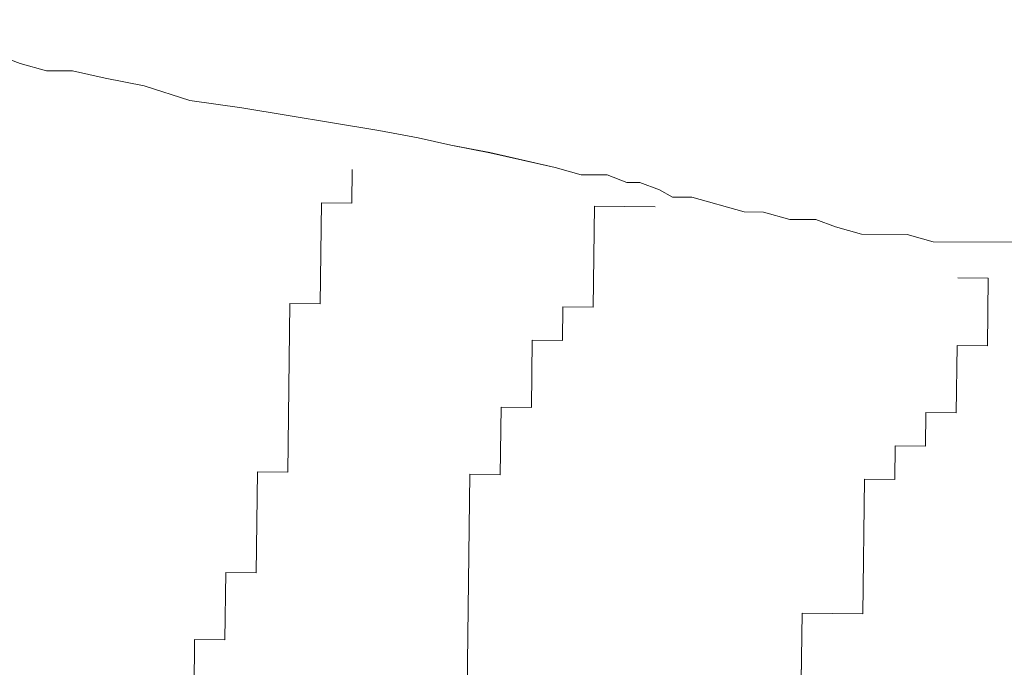
# Model space of a CAD drawing. Units: inches. Extents: x -466983 to 1020, y 324 to 318697.
# Tile 71 of 97: x 643.839 to 647.874, y 945.322 to 947.975. Entities that reach past the tile are written whole.
import ezdxf

# ---------------------------------------------------------------- set-up
doc = ezdxf.new("R2010")
doc.units = ezdxf.units.IN
doc.header["$MEASUREMENT"] = 0
doc.layers.add('A-FLOR-PATT', color=252, linetype='Continuous', lineweight=13)
doc.layers.add('A-FURN', color=8, linetype='Continuous', lineweight=18)

# ---------------------------------------------------------------- blocks, each defined once
blk = doc.blocks.new('L Shaped Sofa')
at = {"ltscale": 2}
for p, q in [((2415.2897, 737.5028), (2415.3174, 739.77)), ((2417.3467, 738.7374), (2417.3559, 739.4931)), ((2412.8069, 738.5409), (2412.813, 739.0447)), ((2417.1137, 738.2363), (2417.1198, 738.7401)), ((2417.1198, 738.7401), (2417.3467, 738.7374)), ((2412.3409, 737.5388), (2412.3532, 738.5464)), ((2412.3532, 738.5464), (2412.8069, 738.5409)), ((2416.8776, 737.4834), (2416.8868, 738.2391)), ((2416.8868, 738.2391), (2417.1137, 738.2363)), ((2412.111, 737.2896), (2412.114, 737.5416)), ((2412.114, 737.5416), (2412.3409, 737.5388)), ((2415.0568, 737.0017), (2415.0629, 737.5055)), ((2415.0629, 737.5055), (2415.2897, 737.5028)), ((2416.6354, 736.2266), (2416.6508, 737.4861)), ((2416.6508, 737.4861), (2416.8776, 737.4834)), ((2411.881, 737.0405), (2411.8841, 737.2924)), ((2411.8841, 737.2924), (2412.111, 737.2896)), ((2411.6481, 736.5394), (2411.6542, 737.0433)), ((2411.6542, 737.0433), (2411.881, 737.0405)), ((2414.8238, 736.5006), (2414.8299, 737.0045)), ((2414.8299, 737.0045), (2415.0568, 737.0017)), ((2411.4151, 736.0384), (2411.4212, 736.5422)), ((2411.4212, 736.5422), (2411.6481, 736.5394)), ((2414.5938, 736.2515), (2414.5969, 736.5034)), ((2414.5969, 736.5034), (2414.8238, 736.5006)), ((2414.3578, 735.4985), (2414.367, 736.2543)), ((2414.367, 736.2543), (2414.5938, 736.2515)), ((2416.3993, 735.4736), (2416.4085, 736.2293)), ((2416.4085, 736.2293), (2416.6354, 736.2266)), ((2411.6419, 736.0356), (2411.4151, 736.0384)), ((2410.4113, 735.7723), (2411.8264, 735.7657)), ((2411.8264, 735.7657), (2412.0212, 735.7106)), ((2412.0212, 735.7106), (2412.3628, 735.709)), ((2412.3628, 735.709), (2412.5576, 735.6538)), ((2412.5576, 735.6538), (2412.7037, 735.5989)), ((2412.7037, 735.5989), (2412.8989, 735.598)), ((2412.8989, 735.598), (2413.0937, 735.5429)), ((2413.0937, 735.5429), (2413.2401, 735.5422)), ((2413.2401, 735.5422), (2413.6298, 735.4319)), ((2413.9041, 735.5041), (2414.3578, 735.4985)), ((2416.1694, 735.2245), (2416.1725, 735.4764)), ((2416.1725, 735.4764), (2416.3993, 735.4736)), ((2413.6298, 735.4319), (2413.7762, 735.4312)), ((2413.7762, 735.4312), (2413.8734, 735.3766)), ((2413.8734, 735.3766), (2414.0195, 735.3217)), ((2414.0195, 735.3217), (2414.1171, 735.3212)), ((2414.1171, 735.3212), (2414.2631, 735.2663)), ((2414.2631, 735.2663), (2414.4583, 735.2654)), ((2414.4583, 735.2654), (2414.6532, 735.2103)), ((2414.6532, 735.2103), (2415.1404, 735.0995)), ((2415.1404, 735.0995), (2415.4329, 735.0439)), ((2415.4329, 735.0439), (2415.6765, 734.9886)), ((2415.6765, 734.9886), (2415.969, 734.933)), ((2415.969, 734.933), (2416.9927, 734.7655)), ((2416.9927, 734.7655), (2417.3827, 734.7095)), ((2417.3827, 734.7095), (2417.7236, 734.5994)), ((2417.7236, 734.5994), (2418.016, 734.5439)), ((2418.016, 734.5439), (2418.2597, 734.4885)), ((2418.2597, 734.4885), (2418.4549, 734.4876)), ((2418.4549, 734.4876), (2418.6497, 734.4324)), ((2418.6497, 734.4324), (2418.7958, 734.3775))]:
    blk.add_line(p, q, dxfattribs=at)

msp = doc.modelspace()

# ---------------------------------------------------------------- hatches: boundary and pattern name
at = {"layer": 'A-FLOR-PATT', "transparency": 33554572}
h = msp.add_hatch(dxfattribs=at)
h.set_pattern_fill('ANSI37', color=256, scale=30)
h.set_pattern_definition([(45, (-1212.4137, -290.035), (-2.6516504, 2.6516504), []), (135, (-1212.4137, -290.035), (-2.6516504, -2.6516504), [])])
h.paths.add_polyline_path([(901.8057, 1075.9377), (900.6144, 1075.9377), (900.6144, 1065.3856), (899.391, 1065.3856), (898.0911, 1065.3856), (892.8356, 1058.7098, -0.258377), (892.1875, 1058.3509), (879.9848, 1058.3509, -0.20177), (879.4382, 1058.5808), (874.0812, 1065.3856), (872.7813, 1065.3856), (871.5579, 1065.3856), (871.5579, 1075.9377), (813.8057, 1075.9377), (813.8057, 1044.7922), (832.3947, 1044.7922, -0.394795), (848.6602, 1028.5356), (848.6602, 1009.9377), (901.8057, 1009.9377), (901.8057, 1015.9377), (901.3057, 1015.9377), (871.3057, 1015.9377), (871.3057, 1017.2502), (871.3344, 1017.2502, -0.401453), (901.3057, 1045.9377), (901.8057, 1045.9377)])
edge = h.paths.add_edge_path(flags=16)
edge.add_line((847.7731, 1068.9486), (847.7731, 1073.7088))
edge.add_arc((849.2269, 1073.7088), 1.4538, 90, 180, ccw=False)
edge.add_line((849.2269, 1075.1627), (864.4921, 1075.1627))
edge.add_arc((864.4921, 1073.7088), 1.4538, 0, 90, ccw=False)
edge.add_line((865.9459, 1073.7088), (865.9459, 1069.0035))
edge.add_arc((832.6447, 1068.9761), 33.3012, -20.61234, 0.04725, ccw=False)
edge.add_ellipse((856.8595, 1058.48), major_axis=(0, 10.2131), ratio=0.6859192, start_angle=100.00884, end_angle=259.99116, ccw=False)
edge.add_arc((881.0742, 1068.9761), 33.3012, 180.04725, 200.61234, ccw=False)
h.paths.add_polyline_path([(853.1456, 1066.4815), (853.1456, 1066.4534), (853.1463, 1066.4534, 0.433107), (852.9166, 1066.6849), (852.9166, 1066.4534), (853.1456, 1066.4534), (853.1456, 1066.4815), (853.088, 1066.6122, 0.697939), (852.6995, 1066.4534), (852.7003, 1066.4534), (852.7003, 1066.4815), (852.9166, 1067.0012), (852.9166, 1066.6849, -0.396254)], flags=0)
h.paths.add_polyline_path([(861.0187, 1066.4815), (861.0187, 1066.4534), (861.0194, 1066.4534, 0.416404), (860.8024, 1066.6849), (860.8024, 1066.4534), (861.0187, 1066.4534), (861.0187, 1066.4815), (860.9672, 1066.6053, 0.713344), (860.5726, 1066.4534), (860.5734, 1066.4534), (860.5734, 1066.4815), (860.8024, 1067.0012), (860.8024, 1066.6849, -0.379973)], flags=0)
edge = h.paths.add_edge_path(flags=0)
edge.add_spline(control_points=[(861.1298, 1065.7855), (861.4661, 1065.2478), (861.6134, 1065.0161), (861.9833, 1064.3736), (862.1924, 1063.9443), (862.5614, 1063.0391), (862.7212, 1062.5633), (862.9865, 1061.5781), (863.092, 1061.0689), (863.2452, 1060.031), (863.293, 1059.5025), (863.3295, 1058.4409), (863.3181, 1057.9078), (863.2366, 1056.8518), (863.1664, 1056.3289), (862.9695, 1055.308), (862.8427, 1054.8099), (862.5365, 1053.8522), (862.3571, 1053.3927), (861.9514, 1052.5249), (861.7251, 1052.1166), (861.233, 1051.3622), (860.9672, 1051.0162), (860.4048, 1050.3949), (860.1082, 1050.1197), (859.4937, 1049.6461), (859.1758, 1049.4476), (858.5276, 1049.1299), (858.1973, 1049.0107), (857.5315, 1048.8518), (857.1959, 1048.8121), (856.5249, 1048.812), (856.1894, 1048.8515), (855.5236, 1049.0101), (855.1933, 1049.1291), (854.545, 1049.4465), (854.2271, 1049.6449), (853.6124, 1050.1183), (853.3158, 1050.3933), (852.7533, 1051.0143), (852.4874, 1051.3602), (851.9952, 1052.1144), (851.7688, 1052.5225), (851.3629, 1053.3902), (851.1834, 1053.8496), (850.877, 1054.8071), (850.7501, 1055.3051), (850.553, 1056.326), (850.4827, 1056.8488), (850.401, 1057.9048), (850.3895, 1058.4379), (850.4257, 1059.4995), (850.4734, 1060.0281), (850.6265, 1061.066), (850.7318, 1061.5753), (850.9969, 1062.5605), (851.1567, 1063.0365), (851.5254, 1063.9418), (851.7345, 1064.3712), (852.1056, 1065.0164), (852.2544, 1065.2503), (852.6082, 1065.7335)], knot_values=[3.915332, 3.915332, 3.915332, 3.915332, 4.013468, 4.013468, 4.175532, 4.175532, 4.337596, 4.337596, 4.49966, 4.49966, 4.661724, 4.661724, 4.823788, 4.823788, 4.985852, 4.985852, 5.147916, 5.147916, 5.30998, 5.30998, 5.472044, 5.472044, 5.634109, 5.634109, 5.796173, 5.796173, 5.958237, 5.958237, 6.120301, 6.120301, 6.282365, 6.282365, 6.444429, 6.444429, 6.606493, 6.606493, 6.768557, 6.768557, 6.930621, 6.930621, 7.092685, 7.092685, 7.254749, 7.254749, 7.416813, 7.416813, 7.578878, 7.578878, 7.740942, 7.740942, 7.903006, 7.903006, 8.06507, 8.06507, 8.227134, 8.227134, 8.389198, 8.389198, 8.551262, 8.551262, 8.65037, 8.65037, 8.65037, 8.65037], degree=3, periodic=0)
edge.add_line((852.6421, 1065.7855), (861.1298, 1065.7855))
edge = h.paths.add_edge_path(flags=0)
edge.add_ellipse((856.8496, 1057.7432), major_axis=(0, 7.7921), ratio=0.687861, start_angle=0, end_angle=360)
h.paths.add_polyline_path([(848.8634, 1069.3891), (848.8634, 1073.9605, -0.414214), (849.9538, 1075.0508), (863.7652, 1075.0508, -0.414214), (864.8555, 1073.9605), (864.8555, 1069.3891, -0.388936), (864.5237, 1069.027, -0.043561), (849.1953, 1069.027, -0.388936)], flags=0)
h.paths.add_polyline_path([(853.1006, 1068.1122, -1), (852.6775, 1068.1122, -1)], flags=0)
edge = h.paths.add_edge_path(flags=0)
edge.add_ellipse((856.8595, 1057.3378), major_axis=(0, 2.207), ratio=0.657164, start_angle=0, end_angle=360)
h.paths.add_polyline_path([(861.0415, 1068.1122, -1), (860.6184, 1068.1122, -1)], flags=0)
edge = h.paths.add_edge_path()
edge.add_line((573.9537, 1057.3412), (573.9537, 1075.9377))
edge.add_line((573.9537, 1075.9377), (558.7308, 1075.9377))
edge.add_line((558.7308, 1075.9377), (558.7308, 1065.3856))
edge.add_line((558.7308, 1065.3856), (557.5074, 1065.3856))
edge.add_line((557.5074, 1065.3856), (556.2075, 1065.3856))
edge.add_line((556.2075, 1065.3856), (550.952, 1058.7098))
edge.add_arc((550.3039, 1059.1155), 0.7646, 270, 327.9483, ccw=False)
edge.add_line((550.3039, 1058.3509), (538.1012, 1058.3509))
edge.add_arc((538.1012, 1059.1155), 0.7646, 224.3704, 270, ccw=False)
edge.add_line((537.5546, 1058.5808), (532.1976, 1065.3856))
edge.add_line((532.1976, 1065.3856), (530.8977, 1065.3856))
edge.add_line((530.8977, 1065.3856), (529.6743, 1065.3856))
edge.add_line((529.6743, 1065.3856), (529.6743, 1075.9377))
edge.add_line((529.6743, 1075.9377), (520.8057, 1075.9377))
edge.add_line((520.8057, 1075.9377), (520.8057, 1045.9377))
edge.add_line((520.8057, 1045.9377), (521.3057, 1045.9377))
edge.add_arc((521.3057, 1015.9377), 30, 2.50749, 90, ccw=False)
edge.add_line((551.277, 1017.2502), (551.3057, 1017.2502))
edge.add_line((551.3057, 1017.2502), (551.3057, 1015.9377))
edge.add_line((551.3057, 1015.9377), (520.8057, 1015.9377))
edge.add_line((520.8057, 1015.9377), (520.8057, 1009.9377))
edge.add_line((520.8057, 1009.9377), (559.1913, 1010.4022))
edge.add_arc((559.1913, 1011.856), 1.4538, 180, 270, ccw=False)
edge.add_line((557.7375, 1011.856), (557.7375, 1016.5613))
edge.add_arc((591.0386, 1016.5888), 33.3012, 159.38766, 180.04725, ccw=False)
edge.add_ellipse((566.8239, 1027.0848), major_axis=(0, 10.2131), ratio=0.6859192, start_angle=280.00884, end_angle=439.99116, ccw=False)
edge.add_arc((542.6091, 1016.5888), 33.3012, 0.04725, 20.61234, ccw=False)
edge.add_line((575.9103, 1016.6162), (575.9103, 1011.856))
edge.add_arc((574.4565, 1011.856), 1.4538, -90, 0, ccw=False)
edge.add_line((574.4565, 1010.4022), (608.8057, 1009.9377))
edge.add_line((608.8057, 1009.9377), (608.8057, 1041.0857))
edge.add_line((608.8057, 1041.0857), (590.2179, 1041.0857))
edge.add_arc((590.775, 1057.9074), 16.8309, 181.92775, 268.10321, ccw=False)
edge = h.paths.add_edge_path()
edge.add_ellipse((494.2443, 583.6204), major_axis=(0, 10.2131), ratio=0.6859192, start_angle=280.00884, end_angle=439.99116, ccw=False)
edge.add_arc((470.0296, 573.1243), 33.3012, 0.04725, 20.61234, ccw=False)
edge.add_line((503.3307, 573.1518), (503.3307, 568.3916))
edge.add_arc((501.8769, 568.3916), 1.4538, -90, 0, ccw=False)
edge.add_line((501.8769, 566.9377), (539.8057, 566.9377))
edge.add_line((539.8057, 566.9377), (539.8057, 572.9377))
edge.add_line((539.8057, 572.9377), (539.3057, 572.9377))
edge.add_line((539.3057, 572.9377), (509.3057, 572.9377))
edge.add_line((509.3057, 572.9377), (509.3057, 574.2502))
edge.add_line((509.3057, 574.2502), (509.3344, 574.2502))
edge.add_arc((539.3057, 572.9377), 30, 90, 177.49251, ccw=False)
edge.add_line((539.3057, 602.9377), (539.8057, 602.9377))
edge.add_line((539.8057, 602.9377), (539.8057, 626.9377))
edge.add_line((539.8057, 626.9377), (531.7718, 626.9377))
edge.add_line((531.7718, 626.9377), (531.7718, 616.3856))
edge.add_line((531.7718, 616.3856), (530.5484, 616.3856))
edge.add_line((530.5484, 616.3856), (529.2485, 616.3856))
edge.add_line((529.2485, 616.3856), (523.7105, 609.3509))
edge.add_line((523.7105, 609.3509), (510.7766, 609.3509))
edge.add_line((510.7766, 609.3509), (505.2386, 616.3856))
edge.add_line((505.2386, 616.3856), (503.9387, 616.3856))
edge.add_line((503.9387, 616.3856), (502.7153, 616.3856))
edge.add_line((502.7153, 616.3856), (502.7153, 626.9377))
edge.add_line((502.7153, 626.9377), (481.6983, 626.9377))
edge.add_line((481.6983, 626.9377), (481.6983, 610.995))
edge.add_arc((467.2703, 611.4728), 14.4359, 271.92775, 358.10321, ccw=False)
edge.add_line((467.7559, 597.0451), (451.8057, 597.0451))
edge.add_line((451.8057, 597.0451), (451.8057, 584.4035))
edge.add_line((451.8057, 584.4035), (451.8057, 566.9377))
edge.add_line((451.8057, 566.9377), (486.6117, 566.9377))
edge.add_arc((486.6117, 568.3916), 1.4538, 180, 270, ccw=False)
edge.add_line((485.1579, 568.3916), (485.1579, 573.0969))
edge.add_arc((518.4591, 573.1243), 33.3012, 159.38766, 180.04725, ccw=False)
h.paths.add_polyline_path([(836.2609, 1020.7328), (879.8898, 1020.7328), (879.8898, 1039.3902), (836.2609, 1039.3902)], flags=25)
h.paths.add_polyline_path([(549.9851, 1036.7492), (593.614, 1036.7492), (593.614, 1055.4065), (549.9851, 1055.4065)], flags=24)
h.paths.add_polyline_path([(475.123, 595.5959), (518.752, 595.5959), (518.752, 614.2532), (475.123, 614.2532)], flags=24)
h = msp.add_hatch(dxfattribs=at)
h.set_pattern_fill('ANSI37', color=256, scale=20)
h.set_pattern_definition([(45, (-1212.4137, -290.035), (-1.767767, 1.767767), []), (135, (-1212.4137, -290.035), (-1.767767, -1.767767), [])])
h.paths.add_polyline_path([(809.8057, 870.9377), (809.8057, 888.1519), (806.9985, 888.1519), (802.6624, 888.1519), (789.3832, 888.1519), (786.2846, 888.1519, -0.414214), (785.4991, 888.9374), (785.4991, 900.1959), (785.4991, 908.4696, -0.414214), (786.8082, 909.7787, -0.414214), (785.4991, 911.0878), (785.4991, 929.1015, -0.414214), (786.8082, 930.4106, -0.414214), (785.4991, 931.7197), (785.4991, 931.9039, -0.414214), (784.19, 930.5948), (766.7223, 930.5948, -0.412359), (765.4132, 931.8956, -0.413741), (764.1145, 930.5782), (744.5781, 930.422, -0.416556), (743.7864, 931.2075), (743.7864, 933.5153), (742.2154, 933.5153), (742.2154, 952.024, -0.001344), (743.7864, 952.1998), (743.7864, 953.9377), (678.5915, 953.9377), (678.5915, 951.1305), (678.5915, 946.7945), (678.5915, 933.5153), (678.5915, 930.4166, -0.414214), (677.806, 929.6312), (666.5475, 929.6312), (658.2738, 929.6312, -0.414214), (656.9647, 930.9403, -0.414214), (655.6556, 929.6312), (637.6419, 929.6312, -0.414214), (636.3328, 930.9403, -0.414214), (635.0237, 929.6312), (634.8395, 929.6312, -0.414214), (636.1486, 928.322), (636.1486, 910.8544, -0.412359), (634.8478, 909.5452, -0.413741), (636.1653, 908.2466), (636.3214, 888.7102, -0.416556), (635.5359, 887.9184), (633.2281, 887.9184), (633.2281, 886.3475), (614.7194, 886.3475, -0.001344), (614.5436, 887.9184), (612.8057, 887.9184), (612.8057, 834.9377), (612.8057, 752.9377), (612.8057, 748.9377), (612.8057, 697.9377), (654.8057, 697.9377), (654.8057, 701.9377), (715.8057, 701.9377), (715.8057, 737.4353), (774.2918, 737.4353), (774.2918, 795.9377), (809.8057, 795.9377)])
h.paths.add_polyline_path([(679.2761, 849.5757, 0.102523), (682.1475, 849.2608, -0.080461), (694.5428, 849.7725, -0.283899), (694.4822, 849.0082, 0.136605), (694.4068, 848.8103, -0.030441), (694.5428, 846.8929), (694.5428, 842.6198), (694.5428, 838.3466, -0.028219), (694.4246, 836.5684), (694.425, 836.5684, 0.196187), (694.4456, 836.2708, -0.302897), (694.5428, 835.467, -0.080461), (682.1475, 835.9787, 0.102523), (679.2761, 835.6638, -0.58611), (678.6457, 836.0169), (678.6457, 849.2227, -0.58611)], flags=16)
h.paths.add_polyline_path([(679.5173, 848.6515, 0.699597), (679.476, 848.6342, 1.20716), (679.1935, 848.7422, 0.010621)], flags=0)
h.paths.add_polyline_path([(679.4923, 836.5608, -0.013798), (679.9178, 836.6594, -0.071703), (682.8533, 837.1434, -0.165743), (682.1665, 839.1006), (682.1665, 842.6094), (682.1665, 846.0603, -0.240616), (683.4733, 848.6767, -0.068263), (693.9295, 849.0082), (693.7875, 848.7083), (693.7875, 849.0228, 0.067332), (683.4733, 848.6767, 0.240616), (682.1665, 846.0603), (682.1665, 842.6094), (682.1665, 839.1006, 0.23459), (683.461, 836.5513, 0.068093), (693.7875, 836.1955), (693.7875, 836.5104), (693.9296, 836.2102, -0.077215), (682.2421, 836.7815, 0.086627), (679.5283, 836.5701, -0.628402), (679.5029, 836.5735), (679.5029, 836.6071, 0.910458)], flags=0)
h.paths.add_polyline_path([(679.476, 848.6364), (679.2069, 848.647), (679.2069, 836.5718, 0.913566), (679.3645, 836.5861), (679.476, 836.5824)], flags=0)
h.paths.add_polyline_path([(679.2761, 829.8604, 0.102523), (682.1475, 829.5455, -0.080461), (694.5428, 830.0572, -0.283899), (694.4822, 829.2929, 0.136605), (694.4068, 829.095, -0.030441), (694.5428, 827.1776), (694.5428, 822.9045), (694.5428, 818.6314, -0.028219), (694.4246, 816.8531), (694.425, 816.8532, 0.196187), (694.4456, 816.5555, -0.302897), (694.5428, 815.7517, -0.080461), (682.1475, 816.2635, 0.102523), (679.2761, 815.9485, -0.58611), (678.6457, 816.3016), (678.6457, 829.5074, -0.58611)], flags=16)
h.paths.add_polyline_path([(679.5173, 828.9362, 0.699597), (679.476, 828.9189, 1.20716), (679.1935, 829.0269, 0.010621)], flags=0)
h.paths.add_polyline_path([(679.4923, 816.8456, -0.013798), (679.9178, 816.9441, -0.071703), (682.8533, 817.4281, -0.165743), (682.1665, 819.3853), (682.1665, 822.8941), (682.1665, 826.345, -0.240616), (683.4733, 828.9614, -0.068263), (693.9295, 829.2929), (693.7875, 828.9931), (693.7875, 829.3076, 0.067332), (683.4733, 828.9614, 0.240616), (682.1665, 826.345), (682.1665, 822.8941), (682.1665, 819.3853, 0.23459), (683.461, 816.836, 0.068093), (693.7875, 816.4802), (693.7875, 816.7952), (693.9296, 816.4949, -0.077215), (682.2421, 817.0662, 0.086627), (679.5283, 816.8549, -0.628402), (679.5029, 816.8582), (679.5029, 816.8918, 0.910458)], flags=0)
h.paths.add_polyline_path([(679.476, 828.9211), (679.2069, 828.9317), (679.2069, 816.8565, 0.913566), (679.3645, 816.8708), (679.476, 816.8671)], flags=0)
h.paths.add_polyline_path([(679.2761, 810.1451, 0.102523), (682.1475, 809.8302, -0.080461), (694.5428, 810.342, -0.3023), (694.4466, 809.5394, 0.10023), (694.4058, 809.3878, -0.03057), (694.5428, 807.4623), (694.5428, 803.1892), (694.5428, 798.9161, -0.03057), (694.4058, 796.9906, 0.10023), (694.4466, 796.839, -0.3023), (694.5428, 796.0365, -0.080461), (682.1475, 796.5482, 0.102523), (679.2761, 796.2333, -0.58611), (678.6457, 796.5863), (678.6457, 809.7921, -0.58611)], flags=16)
h.paths.add_polyline_path([(679.5173, 809.2417, 0.699597), (679.476, 809.2244, 1.20716), (679.1935, 809.3324, 0.010621)], flags=0)
h.paths.add_polyline_path([(679.4923, 797.151, -0.013798), (679.9178, 797.2496, -0.071703), (682.8533, 797.7336, -0.165743), (682.1665, 799.6908), (682.1665, 803.1996), (682.1665, 806.6505, -0.239349), (683.461, 809.2577, -0.072465), (694.4468, 809.5405, 0.197932), (694.425, 809.2405), (693.7875, 809.2985), (693.7875, 809.6135, 0.068093), (683.461, 809.2577, 0.239349), (682.1665, 806.6505), (682.1665, 803.1996), (682.1665, 799.6908, 0.235854), (683.4733, 797.1323, 0.067332), (693.7875, 796.7861), (693.7875, 797.1006), (694.425, 797.1586, 0.197932), (694.4468, 796.8586, -0.080419), (682.1557, 797.3795, 0.083867), (679.5283, 797.1603, -0.628402), (679.5029, 797.1637), (679.5029, 797.1973, 0.910458)], flags=0)
h.paths.add_polyline_path([(679.2069, 809.2372), (679.2069, 797.162, 0.913566), (679.3645, 797.1763), (679.476, 797.1726), (679.476, 809.2266)], flags=0)
h.paths.add_polyline_path([(695.3643, 853.2989), (728.2231, 853.2989), (728.2231, 771.1519), (695.3643, 771.1519)], flags=16)
h.paths.add_polyline_path([(696.0215, 852.6417), (727.5659, 852.6417), (727.5659, 771.809), (696.0215, 771.809)], flags=0)
h.paths.add_polyline_path([(679.2761, 788.7869, 0.102523), (682.1475, 788.472, -0.080461), (694.5428, 788.9837, -0.3023), (694.4466, 788.1812, 0.10023), (694.4058, 788.0296, -0.03057), (694.5428, 786.1041), (694.5428, 781.831), (694.5428, 777.5578, -0.03057), (694.4058, 775.6323, 0.10023), (694.4466, 775.4808, -0.3023), (694.5428, 774.6782, -0.080461), (682.1475, 775.19, 0.102523), (679.2761, 774.875, -0.58611), (678.6457, 775.2281), (678.6457, 788.4339, -0.58611)], flags=16)
h.paths.add_polyline_path([(679.5173, 787.8834, 0.699597), (679.476, 787.8662, 1.20716), (679.1935, 787.9742, 0.010621)], flags=0)
h.paths.add_polyline_path([(679.4923, 775.7928, -0.013798), (679.9178, 775.8914, -0.071703), (682.8533, 776.3753, -0.165743), (682.1665, 778.3325), (682.1665, 781.8414), (682.1665, 785.2922, -0.239349), (683.461, 787.8995, -0.072465), (694.4468, 788.1823, 0.197932), (694.425, 787.8823), (693.7875, 787.9403), (693.7875, 788.2553, 0.068093), (683.461, 787.8995, 0.239349), (682.1665, 785.2922), (682.1665, 781.8414), (682.1665, 778.3325, 0.235854), (683.4733, 775.7741, 0.067332), (693.7875, 775.4279), (693.7875, 775.7424), (694.425, 775.8004, 0.197932), (694.4468, 775.5004, -0.080419), (682.1557, 776.0212, 0.083867), (679.5283, 775.8021, -0.628402), (679.5029, 775.8054), (679.5029, 775.8391, 0.910458)], flags=0)
h.paths.add_polyline_path([(679.2069, 787.8789), (679.2069, 775.8038, 0.913566), (679.3645, 775.818), (679.476, 775.8144), (679.476, 787.8684)], flags=0)
h.paths.add_polyline_path([(704.641, 854.1204, -0.080461), (705.1527, 866.5157, 0.102523), (704.8378, 869.3871, -0.58611), (705.1908, 870.0174), (718.3966, 870.0174, -0.58611), (718.7496, 869.3871, 0.102523), (718.4347, 866.5157, -0.080461), (718.9465, 854.1204, -0.3023), (718.1439, 854.2166, 0.10023), (717.9924, 854.2574, -0.03057), (716.0668, 854.1204), (711.7937, 854.1204), (707.5206, 854.1204, -0.03057), (705.5951, 854.2574, 0.10023), (705.4435, 854.2166, -0.3023)], flags=16)
h.paths.add_polyline_path([(717.8462, 869.1459, 0.699597), (717.8289, 869.1872, 1.20716), (717.9369, 869.4697, 0.010621)], flags=0)
h.paths.add_polyline_path([(705.4631, 854.2164, -0.080419), (705.984, 866.5074, 0.083867), (705.7648, 869.1349, -0.628402), (705.7682, 869.1603), (705.8018, 869.1603, 0.910458), (705.7555, 869.1709, -0.013798), (705.8541, 868.7454, -0.071703), (706.3381, 865.8099, -0.165743), (708.2953, 866.4967), (711.8041, 866.4967), (715.255, 866.4967, -0.239349), (717.8622, 865.2022, -0.072465), (718.145, 854.2164, 0.197932), (717.845, 854.2382), (717.903, 854.8757), (718.218, 854.8757, 0.068093), (717.8622, 865.2022, 0.239349), (715.255, 866.4967), (711.8041, 866.4967), (708.2953, 866.4967, 0.235854), (705.7368, 865.1898, 0.067332), (705.3906, 854.8757), (705.7051, 854.8757), (705.7631, 854.2382, 0.197932)], flags=16)
h.paths.add_polyline_path([(705.7665, 869.4563, 0.913566), (705.7808, 869.2987), (705.7771, 869.1872), (717.8311, 869.1872), (717.8417, 869.4563)], flags=0)
h.paths.add_polyline_path([(729.0446, 842.6198), (729.0446, 846.8929, -0.03057), (729.1817, 848.8184, 0.10023), (729.1408, 848.9699, -0.3023), (729.0446, 849.7725, -0.080461), (741.4399, 849.2608, 0.102523), (744.3113, 849.5757, -0.58611), (744.9417, 849.2227), (744.9417, 836.0169, -0.58611), (744.3113, 835.6638, 0.102523), (741.4399, 835.9787, -0.080461), (729.0446, 835.467, -0.3023), (729.1408, 836.2696, 0.10023), (729.1817, 836.4211, -0.03057), (729.0446, 838.3466)], flags=16)
h.paths.add_polyline_path([(744.1115, 836.5846, 1.20716), (744.3939, 836.4766, 0.010621), (744.0701, 836.5673, 0.699597)], flags=0)
h.paths.add_polyline_path([(729.1407, 836.2684, 0.197932), (729.1624, 836.5684), (729.7999, 836.5104), (729.7999, 836.1955, 0.068093), (740.1264, 836.5513, 0.239349), (741.4209, 839.1585), (741.4209, 842.6094), (741.4209, 846.1182, 0.235854), (740.1141, 848.6767, 0.067332), (729.7999, 849.0228), (729.7999, 848.7083), (729.1624, 848.6503, 0.197932), (729.1407, 848.9504, -0.080419), (741.4317, 848.4295, 0.083867), (744.0591, 848.6486, -0.628402), (744.0845, 848.6453), (744.0845, 848.6117, 0.910458), (744.0951, 848.6579, -0.013798), (743.6696, 848.5594, -0.071703), (740.7341, 848.0754, -0.165743), (741.4209, 846.1182), (741.4209, 842.6094), (741.4209, 839.1585, -0.239349), (740.1264, 836.5513, -0.072465)], flags=0)
h.paths.add_polyline_path([(729.0446, 830.0572, -0.080461), (741.4399, 829.5455, 0.102523), (744.3113, 829.8604, -0.58611), (744.9417, 829.5074), (744.9417, 816.3016, -0.58611), (744.3113, 815.9485, 0.102523), (741.4399, 816.2635, -0.080461), (729.0446, 815.7517, -0.3023), (729.1408, 816.5543, 0.10023), (729.1817, 816.7058, -0.03057), (729.0446, 818.6314), (729.0446, 822.9045), (729.0446, 827.1776, -0.03057), (729.1817, 829.1031, 0.10023), (729.1408, 829.2547, -0.3023)], flags=16)
h.paths.add_polyline_path([(744.1115, 816.8693, 1.20716), (744.3939, 816.7613, 0.010621), (744.0701, 816.852, 0.699597)], flags=0)
h.paths.add_polyline_path([(729.1407, 829.2351, -0.080419), (741.4317, 828.7142, 0.083867), (744.0591, 828.9334, -0.628402), (744.0845, 828.93), (744.0845, 828.8964, 0.910458), (744.0951, 828.9427, -0.013798), (743.6696, 828.8441, -0.071703), (740.7341, 828.3601, -0.165743), (741.4209, 826.4029), (741.4209, 822.8941), (741.4209, 819.4432, -0.239349), (740.1264, 816.836, -0.072465), (729.1407, 816.5531, 0.197932), (729.1624, 816.8532), (729.7999, 816.7952), (729.7999, 816.4802, 0.068093), (740.1264, 816.836, 0.239349), (741.4209, 819.4432), (741.4209, 822.8941), (741.4209, 826.4029, 0.235854), (740.1141, 828.9614, 0.067332), (729.7999, 829.3076), (729.7999, 828.9931), (729.1624, 828.9351, 0.197932)], flags=16)
h.paths.add_polyline_path([(729.0446, 810.342, -0.080461), (741.4399, 809.8302, 0.102523), (744.3113, 810.1451, -0.58611), (744.9417, 809.7921), (744.9417, 796.5863, -0.58611), (744.3113, 796.2333, 0.102523), (741.4399, 796.5482, -0.080461), (729.0446, 796.0365, -0.283899), (729.1052, 796.8007, 0.136605), (729.1806, 796.9987, -0.030441), (729.0446, 798.9161), (729.0446, 803.1892), (729.0446, 807.4623, -0.028219), (729.1628, 809.2406), (729.1624, 809.2405, 0.196187), (729.1418, 809.5382, -0.302897)], flags=16)
h.paths.add_polyline_path([(744.1115, 797.1748, 1.20716), (744.3939, 797.0668, 0.010621), (744.0701, 797.1575, 0.699597)], flags=0)
h.paths.add_polyline_path([(741.3453, 809.0275, 0.086627), (744.0591, 809.2388, -0.628402), (744.0845, 809.2355), (744.0845, 809.2019, 0.910458), (744.0951, 809.2481, -0.013798), (743.6696, 809.1496, -0.071703), (740.7341, 808.6656, -0.165743), (741.4209, 806.7084), (741.4209, 803.1996), (741.4209, 799.7487, -0.240616), (740.1141, 797.1323, -0.068263), (729.658, 796.8008), (729.7999, 797.1006), (729.7999, 796.7861, 0.067332), (740.1141, 797.1323, 0.240616), (741.4209, 799.7487), (741.4209, 803.1996), (741.4209, 806.7084, 0.23459), (740.1264, 809.2577, 0.068093), (729.7999, 809.6135), (729.7999, 809.2985), (729.6578, 809.5988, -0.077215)], flags=0)
h.paths.add_polyline_path([(704.641, 770.3304, -0.283899), (705.4053, 770.2697, 0.136605), (705.6032, 770.1944, -0.030441), (707.5206, 770.3304), (711.7937, 770.3304), (716.0668, 770.3304, -0.028219), (717.8451, 770.2122), (717.845, 770.2126, 0.196187), (718.1427, 770.2331, -0.302897), (718.9465, 770.3304, -0.080461), (718.4347, 757.9351, 0.102523), (718.7496, 755.0637, -0.58611), (718.3966, 754.4333), (705.1908, 754.4333, -0.58611), (704.8378, 755.0637, 0.102523), (705.1527, 757.9351, -0.080461)], flags=16)
h.paths.add_polyline_path([(705.762, 755.3048, 0.699597), (705.7793, 755.2635, 1.20716), (705.6713, 754.9811, 0.010621)], flags=0)
h.paths.add_polyline_path([(705.4053, 769.717), (705.7051, 769.5751), (705.3906, 769.5751, 0.067332), (705.7368, 759.2609, 0.240616), (708.3532, 757.954), (711.8041, 757.954), (715.3129, 757.954, 0.23459), (717.8622, 759.2485, 0.068093), (718.218, 769.5751), (717.903, 769.5751), (718.2033, 769.7172, -0.077215), (717.632, 758.0297, 0.086627), (717.8433, 755.3159, -0.628402), (717.84, 755.2904), (717.8064, 755.2904, 0.910458), (717.8526, 755.2799, -0.013798), (717.7541, 755.7053, -0.071703), (717.2701, 758.6409, -0.165743), (715.3129, 757.954), (711.8041, 757.954), (708.3532, 757.954, -0.240616), (705.7368, 759.2609, -0.068263)], flags=0)
h.paths.add_polyline_path([(729.0446, 788.9837, -0.080461), (741.4399, 788.472, 0.102523), (744.3113, 788.7869, -0.58611), (744.9417, 788.4339), (744.9417, 775.2281, -0.58611), (744.3113, 774.875, 0.102523), (741.4399, 775.19, -0.080461), (729.0446, 774.6782, -0.283899), (729.1052, 775.4425, 0.136605), (729.1806, 775.6405, -0.030441), (729.0446, 777.5578), (729.0446, 781.831), (729.0446, 786.1041, -0.028219), (729.1628, 787.8823), (729.1624, 787.8823, 0.196187), (729.1418, 788.1799, -0.302897)], flags=16)
h.paths.add_polyline_path([(744.1115, 775.8165, 1.20716), (744.3939, 775.7086, 0.010621), (744.0701, 775.7993, 0.699597)], flags=0)
h.paths.add_polyline_path([(741.3453, 787.6692, 0.086627), (744.0591, 787.8806, -0.628402), (744.0845, 787.8773), (744.0845, 787.8437, 0.910458), (744.0951, 787.8899, -0.013798), (743.6696, 787.7913, -0.071703), (740.7341, 787.3074, -0.165743), (741.4209, 785.3502), (741.4209, 781.8414), (741.4209, 778.3905, -0.240616), (740.1141, 775.7741, -0.068263), (729.658, 775.4425), (729.7999, 775.7424), (729.7999, 775.4279, 0.067332), (740.1141, 775.7741, 0.240616), (741.4209, 778.3905), (741.4209, 781.8414), (741.4209, 785.3502, 0.23459), (740.1264, 787.8995, 0.068093), (729.7999, 788.2553), (729.7999, 787.9403), (729.6578, 788.2405, -0.077215)], flags=0)
h.paths.add_polyline_path([(744.1115, 848.6364), (744.1115, 836.5824), (744.3805, 836.5718), (744.3805, 848.647, 0.913566), (744.2229, 848.6327)], flags=0)
h.paths.add_polyline_path([(744.2229, 828.9174), (744.1115, 828.9211), (744.1115, 816.8671), (744.3805, 816.8565), (744.3805, 828.9317, 0.913566)], flags=0)
h.paths.add_polyline_path([(717.8311, 755.2635), (705.7771, 755.2635), (705.7665, 754.9945), (717.8417, 754.9945, 0.913566), (717.8274, 755.1521)], flags=0)
h.paths.add_polyline_path([(744.2229, 809.2229), (744.1115, 809.2266), (744.1115, 797.1726), (744.3805, 797.162), (744.3805, 809.2372, 0.913566)], flags=0)
h.paths.add_polyline_path([(744.1115, 787.8684), (744.1115, 775.8144), (744.3805, 775.8038), (744.3805, 787.8789, 0.913566), (744.2229, 787.8647)], flags=0)
h.paths.add_polyline_path([(678.8774, 877.1228), (737.6127, 877.1228), (737.6127, 899.5116), (678.8774, 899.5116)], flags=24)

# ---------------------------------------------------------------- linework, layer by layer
at = {"layer": 'A-FURN', "ltscale": 2}
for p, q in [((643.8418, 947.7961), (643.7618, 947.8262)), ((643.8418, 947.7961), (643.7618, 947.8262)), ((643.8418, 947.7961), (643.7618, 947.8262)), ((643.8418, 947.7961), (643.7618, 947.8262)), ((643.8418, 947.7961), (643.7618, 947.8262)), ((643.8418, 947.7961), (643.7618, 947.8262)), ((643.9487, 947.7658), (643.8418, 947.7961)), ((643.9487, 947.7658), (643.8418, 947.7961)), ((643.9487, 947.7658), (643.8418, 947.7961)), ((643.9487, 947.7658), (643.8418, 947.7961)), ((643.9487, 947.7658), (643.8418, 947.7961)), ((643.9487, 947.7658), (643.8418, 947.7961)), ((644.0557, 947.7653), (643.9487, 947.7658)), ((644.0557, 947.7653), (643.9487, 947.7658)), ((644.0557, 947.7653), (643.9487, 947.7658)), ((644.0557, 947.7653), (643.9487, 947.7658)), ((644.0557, 947.7653), (643.9487, 947.7658)), ((644.0557, 947.7653), (643.9487, 947.7658)), ((644.1892, 947.735), (644.0557, 947.7653)), ((644.1892, 947.735), (644.0557, 947.7653)), ((644.1892, 947.735), (644.0557, 947.7653)), ((644.1892, 947.735), (644.0557, 947.7653)), ((644.1892, 947.735), (644.0557, 947.7653)), ((644.1892, 947.735), (644.0557, 947.7653)), ((644.3496, 947.7045), (644.1892, 947.735)), ((644.3496, 947.7045), (644.1892, 947.735)), ((644.3496, 947.7045), (644.1892, 947.735)), ((644.3496, 947.7045), (644.1892, 947.735)), ((644.3496, 947.7045), (644.1892, 947.735)), ((644.3496, 947.7045), (644.1892, 947.735)), ((644.5364, 947.6442), (644.3496, 947.7045)), ((644.5364, 947.6442), (644.3496, 947.7045)), ((644.5364, 947.6442), (644.3496, 947.7045)), ((644.5364, 947.6442), (644.3496, 947.7045)), ((644.5364, 947.6442), (644.3496, 947.7045)), ((644.5364, 947.6442), (644.3496, 947.7045)), ((644.7503, 947.6135), (644.5364, 947.6442)), ((644.7503, 947.6135), (644.5364, 947.6442)), ((644.7503, 947.6135), (644.5364, 947.6442)), ((644.7503, 947.6135), (644.5364, 947.6442)), ((644.7503, 947.6135), (644.5364, 947.6442)), ((644.7503, 947.6135), (644.5364, 947.6442)), ((645.3115, 947.5217), (644.7503, 947.6135)), ((645.3115, 947.5217), (644.7503, 947.6135)), ((645.3115, 947.5217), (644.7503, 947.6135)), ((645.3115, 947.5217), (644.7503, 947.6135)), ((645.3115, 947.5217), (644.7503, 947.6135)), ((645.3115, 947.5217), (644.7503, 947.6135)), ((645.4718, 947.4912), (645.3115, 947.5217)), ((645.4718, 947.4912), (645.3115, 947.5217)), ((645.4718, 947.4912), (645.3115, 947.5217)), ((645.4718, 947.4912), (645.3115, 947.5217)), ((645.4718, 947.4912), (645.3115, 947.5217)), ((645.4718, 947.4912), (645.3115, 947.5217)), ((645.6054, 947.4608), (645.4718, 947.4912)), ((645.6054, 947.4608), (645.4718, 947.4912)), ((645.6054, 947.4608), (645.4718, 947.4912)), ((645.6054, 947.4608), (645.4718, 947.4912)), ((645.6054, 947.4608), (645.4718, 947.4912)), ((645.6054, 947.4608), (645.4718, 947.4912)), ((645.7657, 947.4304), (645.6054, 947.4608)), ((645.7657, 947.4304), (645.6054, 947.4608)), ((645.7657, 947.4304), (645.6054, 947.4608)), ((645.7657, 947.4304), (645.6054, 947.4608)), ((645.7657, 947.4304), (645.6054, 947.4608)), ((645.7657, 947.4304), (645.6054, 947.4608)), ((646.0328, 947.3697), (645.7657, 947.4304)), ((646.0328, 947.3697), (645.7657, 947.4304)), ((646.0328, 947.3697), (645.7657, 947.4304)), ((646.0328, 947.3697), (645.7657, 947.4304)), ((646.0328, 947.3697), (645.7657, 947.4304)), ((646.0328, 947.3697), (645.7657, 947.4304)), ((645.2016, 947.3619), (645.1999, 947.2238)), ((645.2016, 947.3619), (645.1999, 947.2238)), ((645.2016, 947.3619), (645.1999, 947.2238)), ((645.2016, 947.3619), (645.1999, 947.2238)), ((645.2016, 947.3619), (645.1999, 947.2238)), ((645.2016, 947.3619), (645.1999, 947.2238)), ((646.1396, 947.3394), (646.0328, 947.3697)), ((646.1396, 947.3394), (646.0328, 947.3697)), ((646.1396, 947.3394), (646.0328, 947.3697)), ((646.1396, 947.3394), (646.0328, 947.3697)), ((646.1396, 947.3394), (646.0328, 947.3697)), ((646.1396, 947.3394), (646.0328, 947.3697)), ((646.2466, 947.3389), (646.1396, 947.3394)), ((646.2466, 947.3389), (646.1396, 947.3394)), ((646.2466, 947.3389), (646.1396, 947.3394)), ((646.2466, 947.3389), (646.1396, 947.3394)), ((646.2466, 947.3389), (646.1396, 947.3394)), ((646.2466, 947.3389), (646.1396, 947.3394)), ((646.3267, 947.3088), (646.2466, 947.3389)), ((646.3267, 947.3088), (646.2466, 947.3389)), ((646.3267, 947.3088), (646.2466, 947.3389)), ((646.3267, 947.3088), (646.2466, 947.3389)), ((646.3267, 947.3088), (646.2466, 947.3389)), ((646.3267, 947.3088), (646.2466, 947.3389)), ((646.3802, 947.3086), (646.3267, 947.3088)), ((646.3802, 947.3086), (646.3267, 947.3088)), ((646.3802, 947.3086), (646.3267, 947.3088)), ((646.3802, 947.3086), (646.3267, 947.3088)), ((646.3802, 947.3086), (646.3267, 947.3088)), ((646.3802, 947.3086), (646.3267, 947.3088)), ((646.4603, 947.2785), (646.3802, 947.3086)), ((646.4603, 947.2785), (646.3802, 947.3086)), ((646.4603, 947.2785), (646.3802, 947.3086)), ((646.4603, 947.2785), (646.3802, 947.3086)), ((646.4603, 947.2785), (646.3802, 947.3086)), ((646.4603, 947.2785), (646.3802, 947.3086)), ((646.5136, 947.2485), (646.4603, 947.2785)), ((646.5136, 947.2485), (646.4603, 947.2785)), ((646.5136, 947.2485), (646.4603, 947.2785)), ((646.5136, 947.2485), (646.4603, 947.2785)), ((646.5136, 947.2485), (646.4603, 947.2785)), ((646.5136, 947.2485), (646.4603, 947.2785)), ((645.0756, 947.2253), (645.0705, 946.811)), ((645.0756, 947.2253), (645.0705, 946.811)), ((645.0756, 947.2253), (645.0705, 946.811)), ((645.0756, 947.2253), (645.0705, 946.811)), ((645.0756, 947.2253), (645.0705, 946.811)), ((645.0756, 947.2253), (645.0705, 946.811)), ((645.1999, 947.2238), (645.0756, 947.2253)), ((645.1999, 947.2238), (645.0756, 947.2253)), ((645.1999, 947.2238), (645.0756, 947.2253)), ((645.1999, 947.2238), (645.0756, 947.2253)), ((645.1999, 947.2238), (645.0756, 947.2253)), ((645.1999, 947.2238), (645.0756, 947.2253)), ((646.1948, 947.2116), (646.1897, 946.7973)), ((646.1948, 947.2116), (646.1897, 946.7973)), ((646.1948, 947.2116), (646.1897, 946.7973)), ((646.1948, 947.2116), (646.1897, 946.7973)), ((646.1948, 947.2116), (646.1897, 946.7973)), ((646.1948, 947.2116), (646.1897, 946.7973)), ((646.4435, 947.2086), (646.1948, 947.2116)), ((646.4435, 947.2086), (646.1948, 947.2116)), ((646.4435, 947.2086), (646.1948, 947.2116)), ((646.4435, 947.2086), (646.1948, 947.2116)), ((646.4435, 947.2086), (646.1948, 947.2116)), ((646.4435, 947.2086), (646.1948, 947.2116)), ((646.5938, 947.2481), (646.5136, 947.2485)), ((646.5938, 947.2481), (646.5136, 947.2485)), ((646.5938, 947.2481), (646.5136, 947.2485)), ((646.5938, 947.2481), (646.5136, 947.2485)), ((646.5938, 947.2481), (646.5136, 947.2485)), ((646.5938, 947.2481), (646.5136, 947.2485)), ((646.8075, 947.1877), (646.5938, 947.2481)), ((646.8075, 947.1877), (646.5938, 947.2481)), ((646.8075, 947.1877), (646.5938, 947.2481)), ((646.8075, 947.1877), (646.5938, 947.2481)), ((646.8075, 947.1877), (646.5938, 947.2481)), ((646.8075, 947.1877), (646.5938, 947.2481)), ((646.8877, 947.1873), (646.8075, 947.1877)), ((646.8877, 947.1873), (646.8075, 947.1877)), ((646.8877, 947.1873), (646.8075, 947.1877)), ((646.8877, 947.1873), (646.8075, 947.1877)), ((646.8877, 947.1873), (646.8075, 947.1877)), ((646.8877, 947.1873), (646.8075, 947.1877)), ((646.9946, 947.1571), (646.8877, 947.1873)), ((646.9946, 947.1571), (646.8877, 947.1873)), ((646.9946, 947.1571), (646.8877, 947.1873)), ((646.9946, 947.1571), (646.8877, 947.1873)), ((646.9946, 947.1571), (646.8877, 947.1873)), ((646.9946, 947.1571), (646.8877, 947.1873)), ((647.1016, 947.1566), (646.9946, 947.1571)), ((647.1016, 947.1566), (646.9946, 947.1571)), ((647.1016, 947.1566), (646.9946, 947.1571)), ((647.1016, 947.1566), (646.9946, 947.1571)), ((647.1016, 947.1566), (646.9946, 947.1571)), ((647.1016, 947.1566), (646.9946, 947.1571)), ((647.1816, 947.1265), (647.1016, 947.1566)), ((647.1816, 947.1265), (647.1016, 947.1566)), ((647.1816, 947.1265), (647.1016, 947.1566)), ((647.1816, 947.1265), (647.1016, 947.1566)), ((647.1816, 947.1265), (647.1016, 947.1566)), ((647.1816, 947.1265), (647.1016, 947.1566)), ((647.2884, 947.0963), (647.1816, 947.1265)), ((647.2884, 947.0963), (647.1816, 947.1265)), ((647.2884, 947.0963), (647.1816, 947.1265)), ((647.2884, 947.0963), (647.1816, 947.1265)), ((647.2884, 947.0963), (647.1816, 947.1265)), ((647.2884, 947.0963), (647.1816, 947.1265)), ((647.4757, 947.0954), (647.2884, 947.0963)), ((647.4757, 947.0954), (647.2884, 947.0963)), ((647.4757, 947.0954), (647.2884, 947.0963)), ((647.4757, 947.0954), (647.2884, 947.0963)), ((647.4757, 947.0954), (647.2884, 947.0963)), ((647.4757, 947.0954), (647.2884, 947.0963)), ((647.5825, 947.0651), (647.4757, 947.0954)), ((647.5825, 947.0651), (647.4757, 947.0954)), ((647.5825, 947.0651), (647.4757, 947.0954)), ((647.5825, 947.0651), (647.4757, 947.0954)), ((647.5825, 947.0651), (647.4757, 947.0954)), ((647.5825, 947.0651), (647.4757, 947.0954)), ((648.3583, 947.0615), (647.5825, 947.0651)), ((648.3583, 947.0615), (647.5825, 947.0651)), ((648.3583, 947.0615), (647.5825, 947.0651)), ((648.3583, 947.0615), (647.5825, 947.0651)), ((648.3583, 947.0615), (647.5825, 947.0651)), ((648.3583, 947.0615), (647.5825, 947.0651)), ((647.6836, 946.9172), (647.808, 946.9156)), ((647.6836, 946.9172), (647.808, 946.9156)), ((647.6836, 946.9172), (647.808, 946.9156)), ((647.6836, 946.9172), (647.808, 946.9156)), ((647.6836, 946.9172), (647.808, 946.9156)), ((647.6836, 946.9172), (647.808, 946.9156)), ((647.808, 946.9156), (647.8046, 946.6394)), ((647.808, 946.9156), (647.8046, 946.6394)), ((647.808, 946.9156), (647.8046, 946.6394)), ((647.808, 946.9156), (647.8046, 946.6394)), ((647.808, 946.9156), (647.8046, 946.6394)), ((647.808, 946.9156), (647.8046, 946.6394)), ((644.9461, 946.8125), (644.9377, 946.122)), ((644.9461, 946.8125), (644.9377, 946.122)), ((644.9461, 946.8125), (644.9377, 946.122)), ((644.9461, 946.8125), (644.9377, 946.122)), ((644.9461, 946.8125), (644.9377, 946.122)), ((644.9461, 946.8125), (644.9377, 946.122)), ((645.0705, 946.811), (644.9461, 946.8125)), ((645.0705, 946.811), (644.9461, 946.8125)), ((645.0705, 946.811), (644.9461, 946.8125)), ((645.0705, 946.811), (644.9461, 946.8125)), ((645.0705, 946.811), (644.9461, 946.8125)), ((645.0705, 946.811), (644.9461, 946.8125)), ((646.0653, 946.7988), (646.0636, 946.6607)), ((646.0653, 946.7988), (646.0636, 946.6607)), ((646.0653, 946.7988), (646.0636, 946.6607)), ((646.0653, 946.7988), (646.0636, 946.6607)), ((646.0653, 946.7988), (646.0636, 946.6607)), ((646.0653, 946.7988), (646.0636, 946.6607)), ((646.1897, 946.7973), (646.0653, 946.7988)), ((646.1897, 946.7973), (646.0653, 946.7988)), ((646.1897, 946.7973), (646.0653, 946.7988)), ((646.1897, 946.7973), (646.0653, 946.7988)), ((646.1897, 946.7973), (646.0653, 946.7988)), ((646.1897, 946.7973), (646.0653, 946.7988)), ((645.9393, 946.6622), (645.9359, 946.386)), ((645.9393, 946.6622), (645.9359, 946.386)), ((645.9393, 946.6622), (645.9359, 946.386)), ((645.9393, 946.6622), (645.9359, 946.386)), ((645.9393, 946.6622), (645.9359, 946.386)), ((645.9393, 946.6622), (645.9359, 946.386)), ((646.0636, 946.6607), (645.9393, 946.6622)), ((646.0636, 946.6607), (645.9393, 946.6622)), ((646.0636, 946.6607), (645.9393, 946.6622)), ((646.0636, 946.6607), (645.9393, 946.6622)), ((646.0636, 946.6607), (645.9393, 946.6622)), ((646.0636, 946.6607), (645.9393, 946.6622)), ((647.6803, 946.641), (647.6769, 946.3648)), ((647.6803, 946.641), (647.6769, 946.3648)), ((647.6803, 946.641), (647.6769, 946.3648)), ((647.6803, 946.641), (647.6769, 946.3648)), ((647.6803, 946.641), (647.6769, 946.3648)), ((647.6803, 946.641), (647.6769, 946.3648)), ((647.8046, 946.6394), (647.6803, 946.641)), ((647.8046, 946.6394), (647.6803, 946.641)), ((647.8046, 946.6394), (647.6803, 946.641)), ((647.8046, 946.6394), (647.6803, 946.641)), ((647.8046, 946.6394), (647.6803, 946.641)), ((647.8046, 946.6394), (647.6803, 946.641)), ((645.8116, 946.3875), (645.8082, 946.1113)), ((645.8116, 946.3875), (645.8082, 946.1113)), ((645.8116, 946.3875), (645.8082, 946.1113)), ((645.8116, 946.3875), (645.8082, 946.1113)), ((645.8116, 946.3875), (645.8082, 946.1113)), ((645.8116, 946.3875), (645.8082, 946.1113)), ((645.9359, 946.386), (645.8116, 946.3875)), ((645.9359, 946.386), (645.8116, 946.3875)), ((645.9359, 946.386), (645.8116, 946.3875)), ((645.9359, 946.386), (645.8116, 946.3875)), ((645.9359, 946.386), (645.8116, 946.3875)), ((645.9359, 946.386), (645.8116, 946.3875)), ((647.5525, 946.3663), (647.5508, 946.2282)), ((647.5525, 946.3663), (647.5508, 946.2282)), ((647.5525, 946.3663), (647.5508, 946.2282)), ((647.5525, 946.3663), (647.5508, 946.2282)), ((647.5525, 946.3663), (647.5508, 946.2282)), ((647.5525, 946.3663), (647.5508, 946.2282)), ((647.6769, 946.3648), (647.5525, 946.3663)), ((647.6769, 946.3648), (647.5525, 946.3663)), ((647.6769, 946.3648), (647.5525, 946.3663)), ((647.6769, 946.3648), (647.5525, 946.3663)), ((647.6769, 946.3648), (647.5525, 946.3663)), ((647.6769, 946.3648), (647.5525, 946.3663)), ((647.4265, 946.2297), (647.4248, 946.0916)), ((647.4265, 946.2297), (647.4248, 946.0916)), ((647.4265, 946.2297), (647.4248, 946.0916)), ((647.4265, 946.2297), (647.4248, 946.0916)), ((647.4265, 946.2297), (647.4248, 946.0916)), ((647.4265, 946.2297), (647.4248, 946.0916)), ((647.5508, 946.2282), (647.4265, 946.2297)), ((647.5508, 946.2282), (647.4265, 946.2297)), ((647.5508, 946.2282), (647.4265, 946.2297)), ((647.5508, 946.2282), (647.4265, 946.2297)), ((647.5508, 946.2282), (647.4265, 946.2297)), ((647.5508, 946.2282), (647.4265, 946.2297)), ((644.8133, 946.1235), (644.8083, 945.7092)), ((644.8133, 946.1235), (644.8083, 945.7092)), ((644.8133, 946.1235), (644.8083, 945.7092)), ((644.8133, 946.1235), (644.8083, 945.7092)), ((644.8133, 946.1235), (644.8083, 945.7092)), ((644.8133, 946.1235), (644.8083, 945.7092)), ((644.9377, 946.122), (644.8133, 946.1235)), ((644.9377, 946.122), (644.8133, 946.1235)), ((644.9377, 946.122), (644.8133, 946.1235)), ((644.9377, 946.122), (644.8133, 946.1235)), ((644.9377, 946.122), (644.8133, 946.1235)), ((644.9377, 946.122), (644.8133, 946.1235)), ((645.6838, 946.1129), (645.6686, 944.8699)), ((645.6838, 946.1129), (645.6686, 944.8699)), ((645.6838, 946.1129), (645.6686, 944.8699)), ((645.6838, 946.1129), (645.6686, 944.8699)), ((645.6838, 946.1129), (645.6686, 944.8699)), ((645.6838, 946.1129), (645.6686, 944.8699)), ((645.8082, 946.1113), (645.6838, 946.1129)), ((645.8082, 946.1113), (645.6838, 946.1129)), ((645.8082, 946.1113), (645.6838, 946.1129)), ((645.8082, 946.1113), (645.6838, 946.1129)), ((645.8082, 946.1113), (645.6838, 946.1129)), ((645.8082, 946.1113), (645.6838, 946.1129)), ((647.3004, 946.0931), (647.2937, 945.5407)), ((647.3004, 946.0931), (647.2937, 945.5407)), ((647.3004, 946.0931), (647.2937, 945.5407)), ((647.3004, 946.0931), (647.2937, 945.5407)), ((647.3004, 946.0931), (647.2937, 945.5407)), ((647.3004, 946.0931), (647.2937, 945.5407)), ((647.4248, 946.0916), (647.3004, 946.0931)), ((647.4248, 946.0916), (647.3004, 946.0931)), ((647.4248, 946.0916), (647.3004, 946.0931)), ((647.4248, 946.0916), (647.3004, 946.0931)), ((647.4248, 946.0916), (647.3004, 946.0931)), ((647.4248, 946.0916), (647.3004, 946.0931)), ((644.6839, 945.7107), (644.6806, 945.4345)), ((644.6839, 945.7107), (644.6806, 945.4345)), ((644.6839, 945.7107), (644.6806, 945.4345)), ((644.6839, 945.7107), (644.6806, 945.4345)), ((644.6839, 945.7107), (644.6806, 945.4345)), ((644.6839, 945.7107), (644.6806, 945.4345)), ((644.8083, 945.7092), (644.6839, 945.7107)), ((644.8083, 945.7092), (644.6839, 945.7107)), ((644.8083, 945.7092), (644.6839, 945.7107)), ((644.8083, 945.7092), (644.6839, 945.7107)), ((644.8083, 945.7092), (644.6839, 945.7107)), ((644.8083, 945.7092), (644.6839, 945.7107)), ((647.045, 945.5437), (647.0416, 945.2675)), ((647.045, 945.5437), (647.0416, 945.2675)), ((647.045, 945.5437), (647.0416, 945.2675)), ((647.045, 945.5437), (647.0416, 945.2675)), ((647.045, 945.5437), (647.0416, 945.2675)), ((647.045, 945.5437), (647.0416, 945.2675)), ((647.2937, 945.5407), (647.045, 945.5437)), ((647.2937, 945.5407), (647.045, 945.5437)), ((647.2937, 945.5407), (647.045, 945.5437)), ((647.2937, 945.5407), (647.045, 945.5437)), ((647.2937, 945.5407), (647.045, 945.5437)), ((647.2937, 945.5407), (647.045, 945.5437)), ((644.5562, 945.436), (644.5511, 945.0217)), ((644.5562, 945.436), (644.5511, 945.0217)), ((644.5562, 945.436), (644.5511, 945.0217)), ((644.5562, 945.436), (644.5511, 945.0217)), ((644.5562, 945.436), (644.5511, 945.0217)), ((644.5562, 945.436), (644.5511, 945.0217)), ((644.6806, 945.4345), (644.5562, 945.436)), ((644.6806, 945.4345), (644.5562, 945.436)), ((644.6806, 945.4345), (644.5562, 945.436)), ((644.6806, 945.4345), (644.5562, 945.436)), ((644.6806, 945.4345), (644.5562, 945.436)), ((644.6806, 945.4345), (644.5562, 945.436))]:
    msp.add_line(p, q, dxfattribs=at)

# ---------------------------------------------------------------- block references
at = {"layer": 'A-FURN', "xscale": 0.5482153745360612, "yscale": 0.5482153745360612, "zscale": 0.5482153745360612, "rotation": 180}
msp.add_blockref('L Shaped Sofa', (1969.7828, 1350.4232), dxfattribs=at)

doc.saveas('drawing.dxf')
